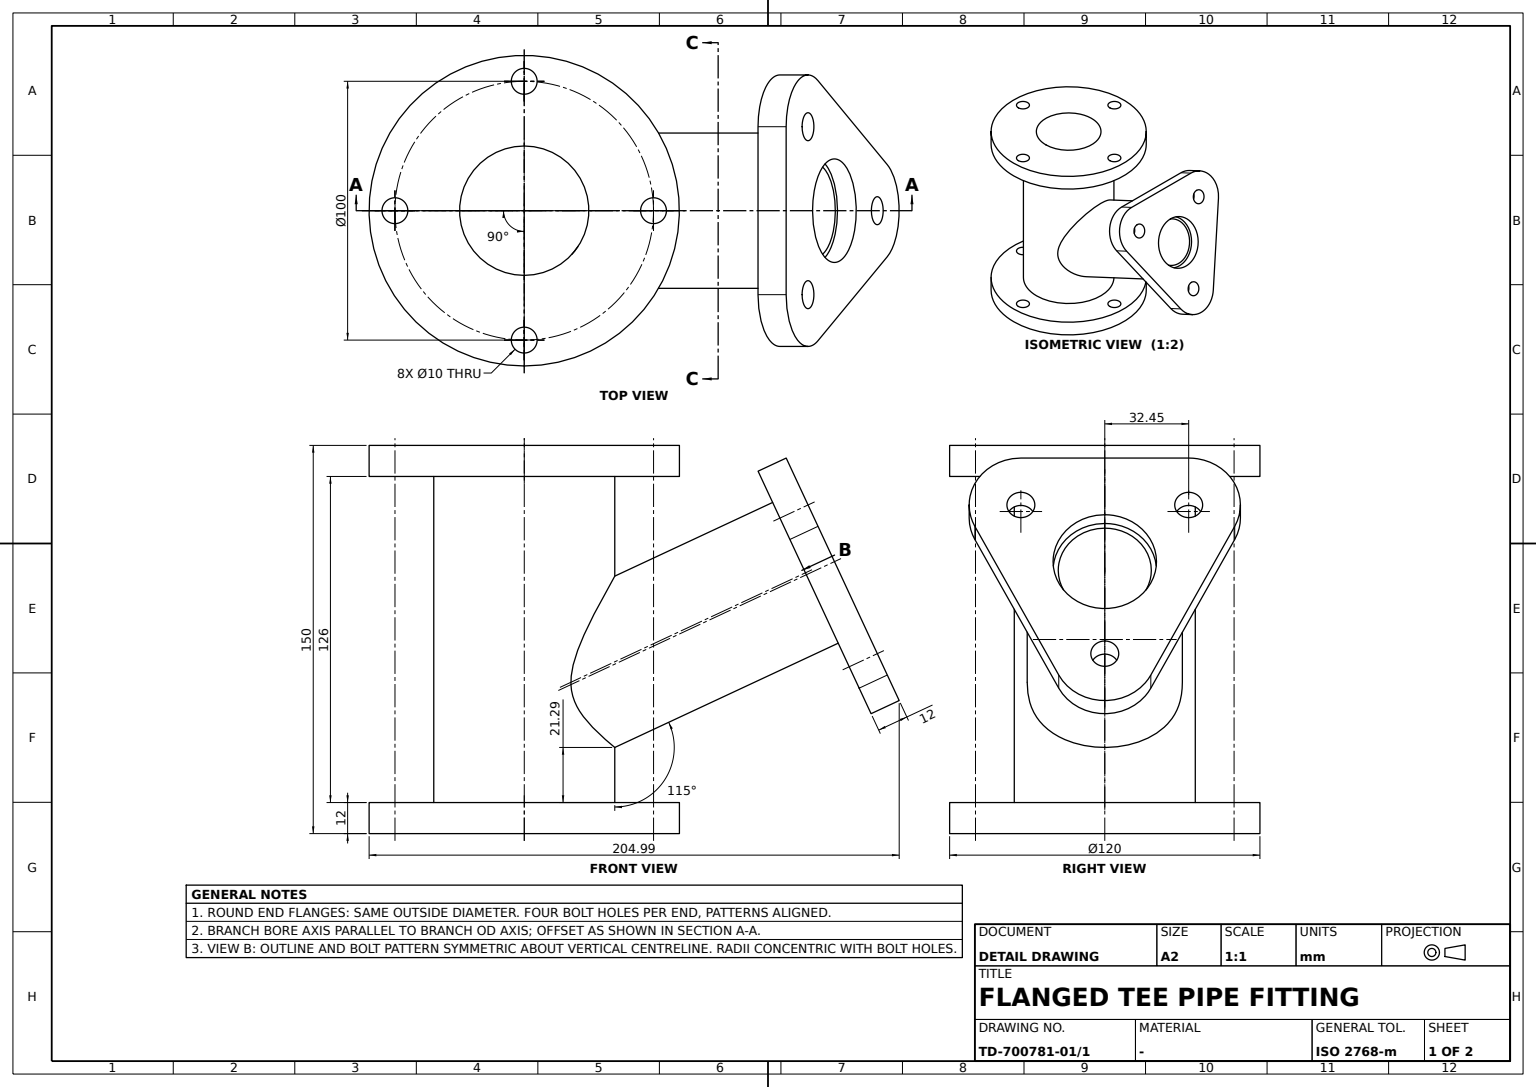
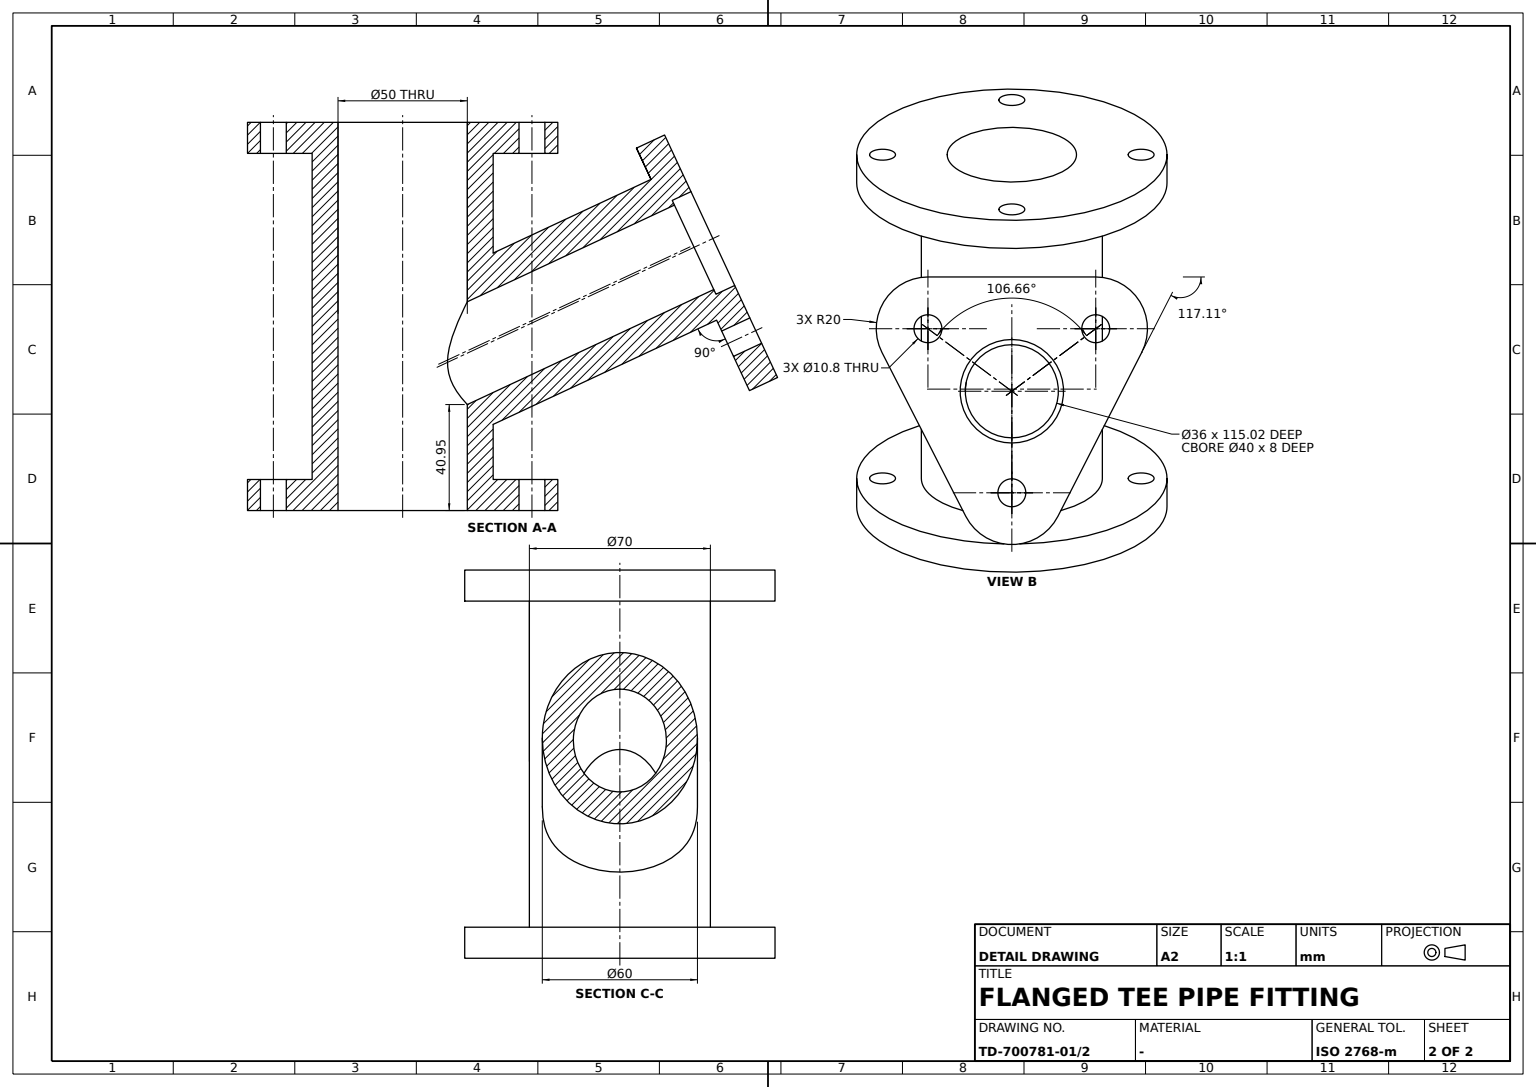
CATIA V5 part; units mm, degrees
sketch "Sketch1" plane through (0, 0, 0) normal (0, 0, 1) x (1, 0, 0)
  circle A0 centre (0, 0) radius 60
  dimension "radius A0" = 60
extrude "Pad1" add sketch "Sketch1" along normal blind 12
sketch "Sketch2" plane through (0, 0, 12) normal (0, 0, 1) x (1, 0, 0)
  circle A0 centre (0, 0) radius 35
  dimension "radius A0" = 35
extrude "Pad2" add sketch "Sketch2" along normal blind 126
sketch "Sketch3" plane through (0, 0, 138) normal (0, 0, 1) x (1, 0, 0)
  circle A0 centre (0, 0) radius 60
  dimension "radius A0" = 60
extrude "Pad3" add sketch "Sketch3" along normal blind 12
sketch "Sketch4" plane through (0, 0, 150) normal (0, 0, 1) x (1, 0, 0)
  circle A0 centre (0, 0) radius 25
  dimension "radius A0" = 25
extrude "Pocket1" cut sketch "Sketch4" against normal blind 150
sketch "Sketch5" plane through (0, 0, 150) normal (0, 0, 1) x (1, 0, 0)
  circle A0 centre (0, 0) radius 50 construction
  circle A1 centre (0, 50) radius 5
  point P0 (0, 50)
  point P1 (0, 45)
  point P2 (-40, 0)
  point P3 (0, -40)
  point P4 (40, 10)
  circle A2 centre (-50, 0) radius 5
  circle A3 centre (0, -50) radius 5
  circle A4 centre (50, 0) radius 5
  dimension "radius A0" = 50
  dimension "radius A1" = 5
  dimension "distance P2 y axis" = 40
  dimension "distance P4 y axis" = 40
  constraint coincidence P0 A0
  constraint coincidence P0 y-axis
  constraint coincidence A1 P1
  constraint coincidence P1 y-axis
extrude "Pocket2" cut sketch "Sketch5" against normal blind 150
ref_plane "Plane1" through (0, 127.908, 59.6445) normal (0, 0.9063, 0.4226) x (-1, 0, 0)
sketch "Sketch8" plane through (0, 127.908, 59.6445) normal (0, 0.9063, 0.4226) x (-1, 0, 0)
  circle A0 centre (0, 45.3741) radius 30
  point P0 (0, 45.3741)
  dimension "radius A0" = 30
  constraint coincidence P0 y-axis
extrude "Pad4" add sketch "Sketch8" against normal up to next
sketch "Sketch9" plane through (0, 127.908, 59.6445) normal (0, 0.9063, 0.4226) x (-1, 0, 0)
  point P0 (0, 45.3154)
  point P1 (0, 45.3154)
  circle A0 centre (0, 45.3154) radius 40 construction
  arc A1 (50.2507, 59.5943) -> (32.4473, 88.7071) centre (32.4473, 68.7071) ccw
  point P2 (32.4473, 68.7071)
  point P3 (16.2237, 57.0112)
  arc A2 (-32.4473, 88.7071) -> (-50.2507, 59.5943) centre (-32.4473, 68.7071) ccw
  point P4 (-32.4473, 68.7071)
  line L0 (-32.4473, 88.7071) -> (32.4473, 88.7071)
  arc A3 (-17.8033, -3.7973) -> (17.8033, -3.7973) centre (0, 5.3154) ccw
  point P5 (0, 5.3154)
  point P6 (0, 25.3154)
  line L1 (17.8033, -3.7973) -> (50.2507, 59.5943)
  line L2 (-17.8033, -3.7973) -> (-50.2507, 59.5943)
  dimension "radius A0" = 40
  constraint coincidence P0 y-axis
  constraint coincidence P0 P1
  constraint coincidence P2 A0
  constraint coincidence A1 P3
  constraint coincidence P4 A0
  constraint coincidence P5 A0
  constraint coincidence P5 y-axis
  constraint coincidence A3 P6
  constraint tangency L0 A2
  constraint tangency L0 A1
  constraint tangency L1 A3
  constraint tangency L1 A1
  constraint tangency L2 A3
  constraint tangency L2 A2
  constraint symmetry A1 A2 y-axis
extrude "Pad5" add sketch "Sketch9" along normal blind 12
sketch "Sketch10" plane through (0, 138.7837, 64.7159) normal (0, 0.9063, 0.4226) x (-1, 0, 0)
  circle A0 centre (0, 44.5474) radius 18
  point P0 (0, 44.5474)
  dimension "radius A0" = 18
  constraint coincidence P0 y-axis
extrude "Pocket3" cut sketch "Sketch10" against normal up to next
sketch "Sketch11" plane through (0, 138.7837, 64.7159) normal (0, 0.9063, 0.4226) x (-1, 0, 0)
  circle A0 centre (0, 44.5474) radius 20
  point P0 (0, 44.5474)
  circle A1 centre (0, 44.5474) radius 18 construction
  dimension "radius A0" = 20
  constraint coincidence P0 y-axis
  constraint concentricity A1 A0
extrude "Pocket4" cut sketch "Sketch11" against normal blind 8
sketch "Sketch12" plane through (0, 138.7837, 64.7159) normal (0, 0.9063, 0.4226) x (-1, 0, 0)
  circle A0 centre (-32.4473, 68.7071) radius 5.4
  circle A1 centre (32.4473, 68.7071) radius 5.4
  circle A2 centre (0, 5.3154) radius 5.4
  arc A3 (50.2507, 59.5943) -> (32.4473, 88.7071) centre (32.4473, 68.7071) ccw construction
  arc A4 (-32.4473, 88.7071) -> (-50.2507, 59.5943) centre (-32.4473, 68.7071) ccw construction
  arc A5 (-17.8033, -3.7973) -> (17.8033, -3.7973) centre (0, 5.3154) ccw construction
  dimension "radius A2" = 5.4
  dimension "radius A1" = 5.4
  dimension "radius A0" = 5.4
  constraint concentricity A1 A3
  constraint concentricity A0 A4
  constraint concentricity A2 A5
extrude "Pocket5" cut sketch "Sketch12" against normal blind 12
sketch "Sketch6" plane through (0, 0, 0) normal (1, 0, 0) x (0, 1, 0)
  line L0 (0, 50) -> (108.7569, 100.7142) construction
  point P0 (0, 50)
  line L1 (-60, 12) -> (60, 12) construction
  dimension "length L0" = 120
  dimension "D2" = 115
  dimension "distance P0 L1" = 38
  constraint coincidence P0 y-axis
sketch "Sketch7" plane through (0, 0, 0) normal (1, 0, 0) x (0, 1, 0)
  line L0 (0, 50) -> (108.7569, 100.7142) construction
  point P0 (0, 50)
  point P1 (108.7569, 100.7142)
  line L1 (45, 12) -> (55, 12) construction
  line L2 (0, 50) -> (108.7569, 100.7142)
  dimension "length L0" = 120
  dimension "distance L1 P0" = 38
  dimension "angle L0 y axis" = 115
  constraint coincidence P0 y-axis
  constraint parallelism L2 L0
